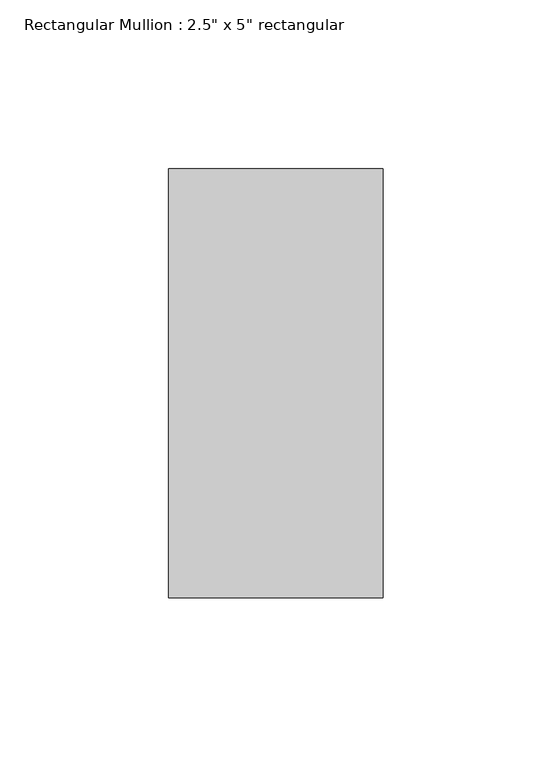
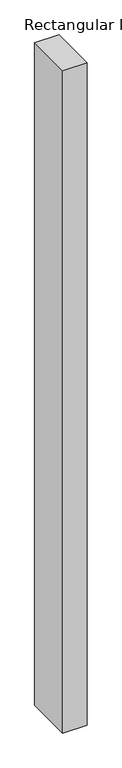
"""IFC4 building model written with IfcOpenShell, lengths in millimetres: member geometry."""

from ifc_helpers import new_model, si_unit, frame, origin, place, context, project, spatial, polyline, outline, extrude, source, transform, mapped, element, save


def member_24f6b202(model_context):
    return source(origin(), model_context, "Body", "SweptSolid", [
        extrude(outline(polyline([(0.0, 63.5), (0.0, -63.5), (-63.5, -63.5), (-63.5, 63.5), (0.0, 63.5)])), frame((0.0, 0.0, -1832.8927429), z_axis=(0.0, 0.0, 1.0), x_axis=(1.0, 0.0, 0.0)), (0.0, 0.0, 1.0), 1832.8927429),
    ])


if __name__ == "__main__":
    model = new_model("IFC4")
    model_context = context("Model", 3, world=origin())
    ifc_project = project(units=[si_unit("LENGTHUNIT", "METRE", prefix="MILLI")], contexts=[model_context])
    site = spatial("IfcSite", under=ifc_project)
    building = spatial("IfcBuilding", under=site)
    placement = place(None, origin())
    member_shape = member_24f6b202(model_context)
    element("IfcMember", 1, ObjectType="Rectangular Mullion : 2.5\" x 5\" rectangular", at=placement, inside=building, context=model_context, shape_type="MappedRepresentation", body=[
        mapped(member_shape, transform((0.0, 0.0, 0.0), x_axis=(1.0, 0.0, 0.0), y_axis=(0.0, 1.0, 0.0), z_axis=(0.0, 0.0, 1.0))),
    ])
    save(model, "model.ifc")

# Revit data of these elements
# Type "Rectangular Mullion : 2.5\" x 5\" rectangular"
#   built-in parameter 1007304 = 0.416667 (stored number, unit not read)
#   built-in parameter 1007301 = 0.104167 (stored number, unit not read)
#   built-in parameter 1007300 = 0.104167 (stored number, unit not read)
# Element 1 (IfcMember, "Rectangular Mullion : 2.5\" x 5\" rectangular")
#   Materials on its faces: "Aluminum"
# Materials
#   "Aluminum": class "Metal", colour RGB 247 247 247, transparency 0, Description = "Aluminum 6061", Cost = 0
